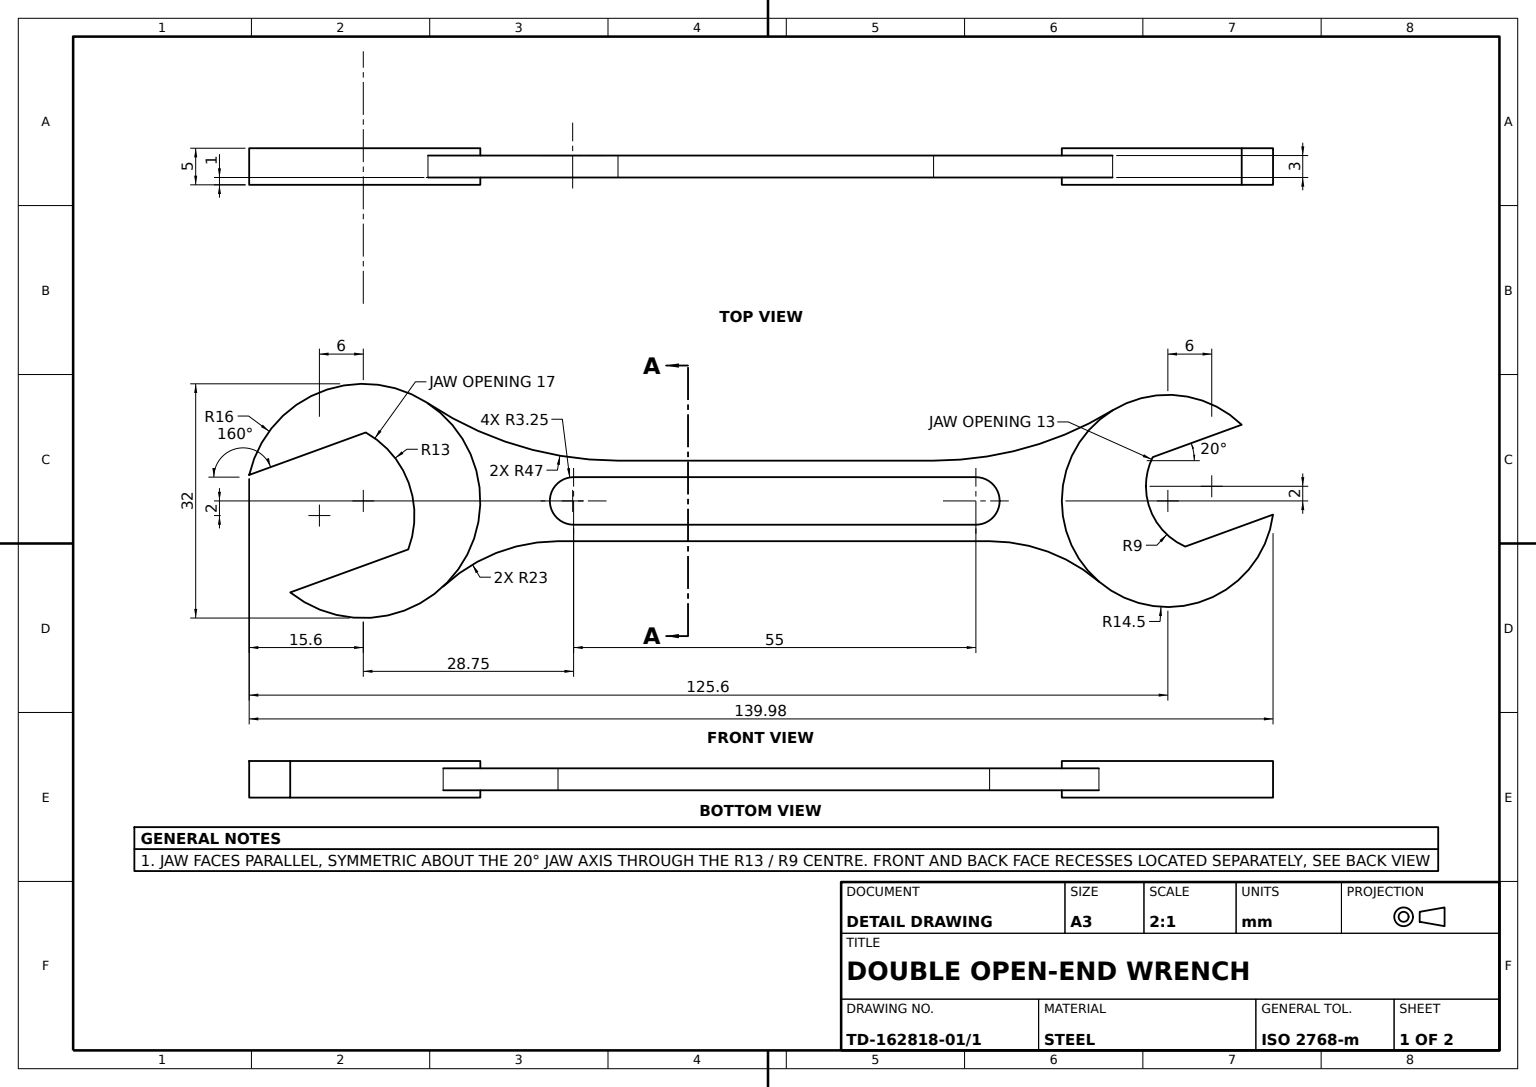
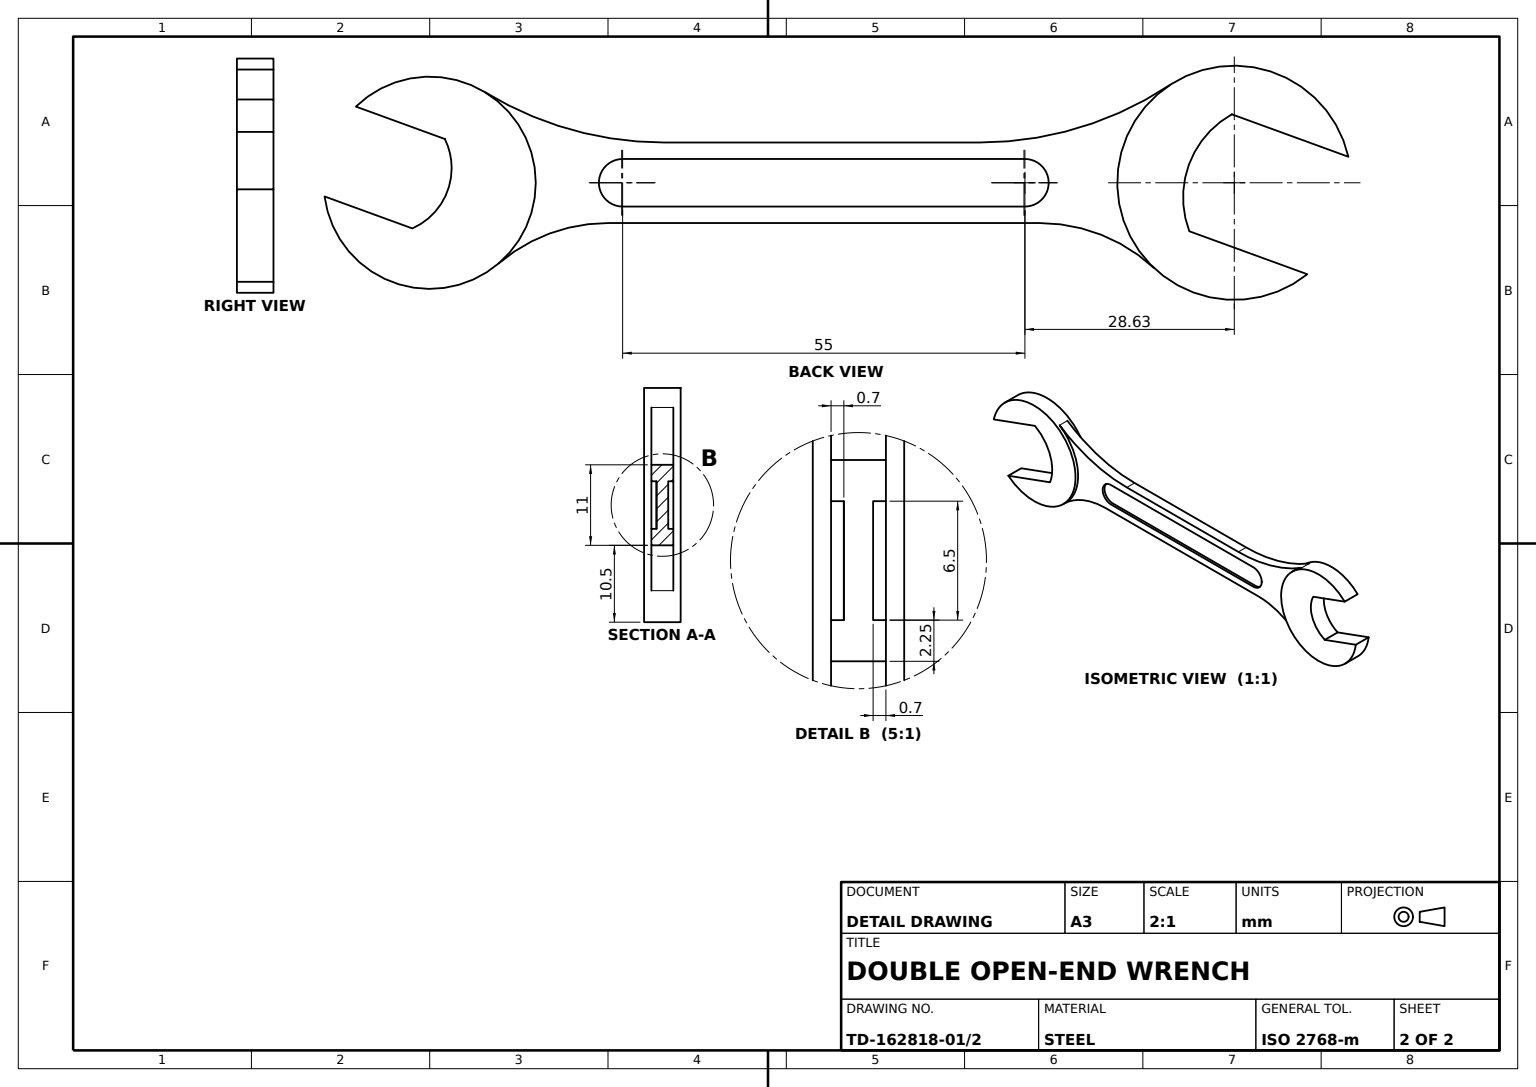
SolidWorks part; units mm, degrees
material "Plain Carbon Steel"
ref_plane "Front Plane" through (0, 0, 0) normal (0, 0, 1) x (1, 0, 0)
ref_plane "Top Plane" through (0, 0, 0) normal (0, 1, 0) x (1, 0, 0)
ref_plane "Right Plane" through (0, 0, 0) normal (1, 0, 0) x (0, 0, -1)
sketch "Spanner Profile Sketch" plane through (0, 0, 0) normal (0, 0, 1) x (1, 0, 0)
  line L0 (0, 0) -> (110, 0)
  line L1 (0, 0) -> (-6, 0)
  line L4 (-6, 0) -> (-6, -2)
  line L7 (-6, -2) -> (-0.505, 0)
  line L8 (110, 0) -> (116, 0)
  line L10 (6.1501, -6.6232) -> (-9.9902, -12.4978)
  line L12 (-15.601, 3.551) -> (0.3358, 9.3516)
  line L13 (34.8246, 5.5) -> (77.9688, 5.5)
  line L14 (26.6224, -5.5) -> (85.6279, -5.5)
  line L16 (120.0958, 10.4079) -> (107.9273, 5.9789)
  line L18 (112.3736, -6.2371) -> (124.3793, -1.8674)
  arc A0 (8.8443, 13.3333) -> (-15.601, 3.551) centre (0, 0) ccw
  arc A1 (100.5761, -11.02) -> (124.3793, -1.8674) centre (110, 0) ccw
  arc A2 (34.8246, 5.5) -> (8.8443, 13.3333) centre (34.8246, 52.5) cw
  arc A3 (102.4479, 12.378) -> (77.9688, 5.5) centre (77.9688, 52.5) cw
  arc A4 (100.5761, -11.02) -> (85.6279, -5.5) centre (85.6279, -28.5) ccw
  arc A5 (26.6224, -5.5) -> (10.922, -11.6923) centre (26.6224, -28.5) ccw
  arc A7 (6.1501, -6.6232) -> (0.3358, 9.3516) centre (-6, -2) ccw
  arc A8 (-9.9902, -12.4978) -> (10.922, -11.6923) centre (0, 0) ccw
  arc A9 (107.9273, 5.9789) -> (112.3736, -6.2371) centre (116, 2) ccw
  arc A10 (120.0958, 10.4079) -> (102.4479, 12.378) centre (110, 0) ccw
  dimension "D1" = 16
  dimension "D3" = 14.5
  dimension "D2" = 47
  dimension "D4" = 47
  dimension "D5" = 23
  dimension "D8" = 6
  dimension "D11" = 9
  dimension "D13" = 13
  dimension "D20" = 42.127
  dimension "D22" = 8.6727
  dimension "D6" = 6
  dimension "D7" = 2
  dimension "D9" = 20
  dimension "D10" = 2
  dimension "D12" = 17
  dimension "D14" = 13.3333
  dimension "D15" = 11
  dimension "D16" = 15.9368
  dimension "D17" = 21.7511
  dimension "D18" = 125.9902
  dimension "D19" = 38.7514
  dimension "D21" = 12.216
  dimension "D23" = 67.0468
  dimension "D24" = 16.52
  dimension "D25" = 5.5
  dimension "D26" = 15.7004
extrude "Spanner Body 3mm" add sketch "Spanner Profile Sketch" along normal blind 3 contours L16 A10 A3 L13 A2 A0 L12 A7 L0 A9 | A9 L0 A7 L10 A8 A5 L14 A4 A1 L18
sketch "Head Pad 13 Side A Sketch" plane through (0, 0, 3) normal (0, 0, 1) x (1, 0, 0)
  line L0 (-15.601, 3.551) -> (0.3358, 9.3516)
  line L1 (-9.9902, -12.4978) -> (6.1501, -6.6232)
  arc A0 (-9.9902, -12.4978) -> (-15.601, 3.551) centre (0, 0) ccw
  arc A1 (0.3358, 9.3516) -> (6.1501, -6.6232) centre (-6, -2) cw
  dimension "D1" = 13
extrude "Head Pad 13 Side A" add sketch "Head Pad 13 Side A Sketch" along normal blind 1
sketch "Head Pad 13 Side B Sketch" plane through (0, 0, 0) normal (0, 0, -1) x (-1, 0, 0)
  line L0 (-0.3358, 9.3516) -> (15.601, 3.551)
  line L1 (-6.1501, -6.6232) -> (9.9902, -12.4978)
  arc A0 (15.601, 3.551) -> (9.9902, -12.4978) centre (0, 0) ccw
  arc A1 (-6.1501, -6.6232) -> (-0.3358, 9.3516) centre (6, -2) cw
  dimension "D1" = 13
extrude "Head Pad 13 Side B" add sketch "Head Pad 13 Side B Sketch" along normal blind 1
sketch "Head Pad 9 Side A Sketch" plane through (0, 0, 0) normal (0, 0, -1) x (-1, 0, 0)
  line L0 (-107.9273, 5.9789) -> (-120.0958, 10.4079)
  line L1 (-112.3736, -6.2371) -> (-124.3793, -1.8674)
  arc A0 (-124.3793, -1.8674) -> (-120.0958, 10.4079) centre (-110, 0) ccw
  arc A1 (-107.9273, 5.9789) -> (-112.3736, -6.2371) centre (-116, 2) cw
  dimension "D1" = 9
extrude "Head Pad 9 Side A" add sketch "Head Pad 9 Side A Sketch" along normal blind 1
sketch "Head Pad 9 Side B Sketch" plane through (0, 0, 3) normal (0, 0, 1) x (1, 0, 0)
  line L0 (107.9273, 5.9789) -> (120.0958, 10.4079)
  line L1 (112.3736, -6.2371) -> (124.3793, -1.8674)
  arc A0 (120.0958, 10.4079) -> (124.3793, -1.8674) centre (110, 0) ccw
  arc A1 (107.9273, 5.9789) -> (112.3736, -6.2371) centre (116, 2) ccw
  dimension "D1" = 9
extrude "Head Pad 9 Side B" add sketch "Head Pad 9 Side B Sketch" along normal blind 1
sketch "Handle Slot Side A Sketch" plane through (0, 0, 3) normal (0, 0, 1) x (1, 0, 0)
  line L3 (28.7537, 0) -> (83.7537, 0) construction
  line L5 (28.7681, 3.25) -> (83.7537, 3.25)
  line L7 (83.7537, -3.25) -> (28.7537, -3.25)
  arc A0 (28.7681, 3.25) -> (28.7537, -3.25) centre (28.7537, 0) ccw
  arc A1 (83.7537, -3.25) -> (83.7537, 3.25) centre (83.7537, 0) ccw
  point P13 (28.7537, 0)
  dimension "D3" = 3.25
  dimension "D4" = 3.25
  dimension "D5" = 3.25
  dimension "D6" = 28.7537
  dimension "D1" = 55
  dimension "D2" = 6.5
extrude "Handle Slot Side A 55x6.5" cut sketch "Handle Slot Side A Sketch" against normal blind 0.7
sketch "Handle Slot Side B Sketch" plane through (0, 0, 0) normal (0, 0, -1) x (-1, 0, 0)
  line L3 (-56.1251, 0) -> (-28.6251, 0) construction
  line L4 (-56.1251, 0) -> (-83.6251, 0) construction
  line L5 (-83.6251, 3.25) -> (-28.6251, 3.25)
  line L6 (-83.6251, -3.25) -> (-28.6251, -3.25)
  arc A0 (-83.6251, 3.25) -> (-83.6251, -3.25) centre (-83.6251, 0) ccw
  arc A1 (-28.6251, -3.25) -> (-28.6251, 3.25) centre (-28.6251, 0) ccw
  dimension "D1" = 27.5
  dimension "D3" = 3.25
  dimension "D4" = 3.25
  dimension "D2" = 27.5
  dimension "D5" = 55
  dimension "D6" = 55
  dimension "D7" = 56.1251
extrude "Handle Slot Side B 55x6.5" cut sketch "Handle Slot Side B Sketch" against normal blind 0.7
